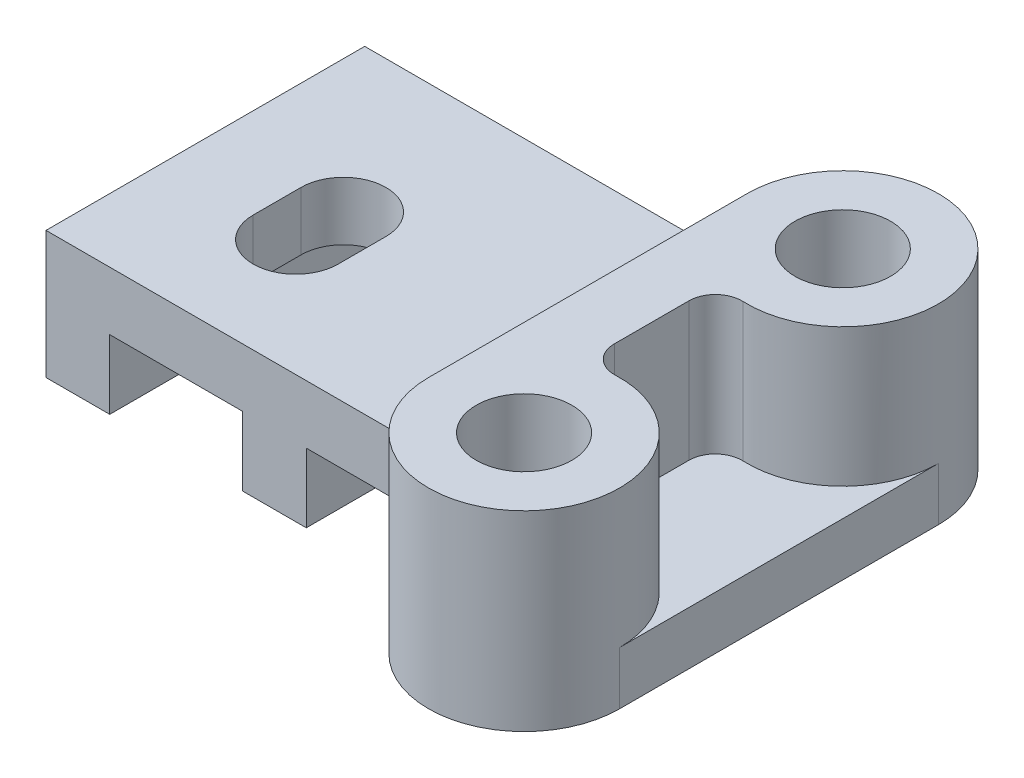
ISO-10303-21;
HEADER;
FILE_DESCRIPTION(('STEP AP214'),'2;1');
FILE_NAME('part.step','',(''),(''),'','','');
FILE_SCHEMA(('AUTOMOTIVE_DESIGN { 1 0 10303 214 1 1 1 1 }'));
ENDSEC;
DATA;
#1=APPLICATION_CONTEXT('core data for automotive mechanical design processes');
#2=APPLICATION_PROTOCOL_DEFINITION('international standard','automotive_design',2000,#1);
#3=PRODUCT_CONTEXT('',#1,'mechanical');
#4=PRODUCT('Part','Part','',(#3));
#5=PRODUCT_RELATED_PRODUCT_CATEGORY('part','',(#4));
#6=PRODUCT_DEFINITION_FORMATION('','',#4);
#7=PRODUCT_DEFINITION_CONTEXT('part definition',#1,'design');
#8=PRODUCT_DEFINITION('design','',#6,#7);
#9=PRODUCT_DEFINITION_SHAPE('','',#8);
#10=(LENGTH_UNIT() NAMED_UNIT(*) SI_UNIT(.MILLI.,.METRE.));
#11=(NAMED_UNIT(*) PLANE_ANGLE_UNIT() SI_UNIT($,.RADIAN.));
#12=(NAMED_UNIT(*) SI_UNIT($,.STERADIAN.) SOLID_ANGLE_UNIT());
#13=UNCERTAINTY_MEASURE_WITH_UNIT(LENGTH_MEASURE(1.E-05),#10,'distance_accuracy_value','');
#14=(GEOMETRIC_REPRESENTATION_CONTEXT(3) GLOBAL_UNCERTAINTY_ASSIGNED_CONTEXT((#13)) GLOBAL_UNIT_ASSIGNED_CONTEXT((#10,
#11,#12)) REPRESENTATION_CONTEXT('',''));
#15=CARTESIAN_POINT('',(0.,0.,0.));
#16=DIRECTION('',(0.,0.,1.));
#17=DIRECTION('',(1.,0.,0.));
#18=AXIS2_PLACEMENT_3D('',#15,#16,#17);
#19=CARTESIAN_POINT('',(90.,0.,0.));
#20=DIRECTION('',(0.,1.,0.));
#21=DIRECTION('',(0.,0.,1.));
#22=AXIS2_PLACEMENT_3D('',#19,#20,#21);
#23=CYLINDRICAL_SURFACE('',#22,18.);
#24=CARTESIAN_POINT('',(90.,10.,0.));
#25=DIRECTION('',(0.,1.,0.));
#26=DIRECTION('',(0.,0.,1.));
#27=AXIS2_PLACEMENT_3D('',#24,#25,#26);
#28=CIRCLE('',#27,18.);
#29=CARTESIAN_POINT('',(89.2173913043478,10.,17.9829787195973));
#30=VERTEX_POINT('',#29);
#31=CARTESIAN_POINT('',(108.,10.,0.));
#32=VERTEX_POINT('',#31);
#33=EDGE_CURVE('E236',#30,#32,#28,.T.);
#34=ORIENTED_EDGE('',*,*,#33,.T.);
#35=DIRECTION('',(0.,-1.,0.));
#36=VECTOR('',#35,1.);
#37=CARTESIAN_POINT('',(108.,10.,0.));
#38=LINE('',#37,#36);
#39=CARTESIAN_POINT('',(108.,0.,0.));
#40=VERTEX_POINT('',#39);
#41=EDGE_CURVE('E244',#32,#40,#38,.T.);
#42=ORIENTED_EDGE('',*,*,#41,.T.);
#43=CARTESIAN_POINT('',(90.,0.,0.));
#44=DIRECTION('',(0.,1.,0.));
#45=DIRECTION('',(0.,0.,1.));
#46=AXIS2_PLACEMENT_3D('',#43,#44,#45);
#47=CIRCLE('',#46,18.);
#48=CARTESIAN_POINT('',(72.,0.,0.));
#49=VERTEX_POINT('',#48);
#50=EDGE_CURVE('E264',#40,#49,#47,.T.);
#51=ORIENTED_EDGE('',*,*,#50,.T.);
#52=DIRECTION('',(0.,1.,0.));
#53=VECTOR('',#52,1.);
#54=CARTESIAN_POINT('',(72.,0.,0.));
#55=LINE('',#54,#53);
#56=CARTESIAN_POINT('',(72.,13.,0.));
#57=VERTEX_POINT('',#56);
#58=EDGE_CURVE('E303',#49,#57,#55,.T.);
#59=ORIENTED_EDGE('',*,*,#58,.T.);
#60=DIRECTION('',(0.,1.,0.));
#61=VECTOR('',#60,1.);
#62=CARTESIAN_POINT('',(72.,13.,0.));
#63=LINE('',#62,#61);
#64=CARTESIAN_POINT('',(72.,24.,0.));
#65=VERTEX_POINT('',#64);
#66=EDGE_CURVE('E344',#57,#65,#63,.T.);
#67=ORIENTED_EDGE('',*,*,#66,.T.);
#68=CARTESIAN_POINT('',(72.,36.,0.));
#69=VERTEX_POINT('',#68);
#70=EDGE_CURVE('E272',#65,#69,#55,.T.);
#71=ORIENTED_EDGE('',*,*,#70,.T.);
#72=CARTESIAN_POINT('',(90.,36.,0.));
#73=DIRECTION('',(0.,1.,0.));
#74=DIRECTION('',(0.,0.,1.));
#75=AXIS2_PLACEMENT_3D('',#72,#73,#74);
#76=CIRCLE('',#75,18.);
#77=CARTESIAN_POINT('',(89.2173913043478,36.,17.9829787195973));
#78=VERTEX_POINT('',#77);
#79=EDGE_CURVE('E265',#78,#69,#76,.T.);
#80=ORIENTED_EDGE('',*,*,#79,.F.);
#81=DIRECTION('',(0.,1.,0.));
#82=VECTOR('',#81,1.);
#83=CARTESIAN_POINT('',(89.2173913043478,0.,17.9829787195973));
#84=LINE('',#83,#82);
#85=EDGE_CURVE('E289',#30,#78,#84,.T.);
#86=ORIENTED_EDGE('',*,*,#85,.F.);
#87=EDGE_LOOP('',(#34,#42,#51,#59,#67,#71,#80,#86));
#88=FACE_BOUND('',#87,.T.);
#89=ADVANCED_FACE('F43',(#88),#23,.T.);
#90=CARTESIAN_POINT('',(0.,24.,60.));
#91=DIRECTION('',(1.,0.,0.));
#92=DIRECTION('',(0.,1.,0.));
#93=AXIS2_PLACEMENT_3D('',#90,#91,#92);
#94=PLANE('',#93);
#95=DIRECTION('',(0.,-1.,0.));
#96=VECTOR('',#95,1.);
#97=CARTESIAN_POINT('',(0.,24.,0.));
#98=LINE('',#97,#96);
#99=CARTESIAN_POINT('',(0.,24.,0.));
#100=VERTEX_POINT('',#99);
#101=CARTESIAN_POINT('',(0.,0.,0.));
#102=VERTEX_POINT('',#101);
#103=EDGE_CURVE('E295',#100,#102,#98,.T.);
#104=ORIENTED_EDGE('',*,*,#103,.T.);
#105=DIRECTION('',(0.,0.,-1.));
#106=VECTOR('',#105,1.);
#107=CARTESIAN_POINT('',(0.,0.,60.));
#108=LINE('',#107,#106);
#109=CARTESIAN_POINT('',(0.,0.,60.));
#110=VERTEX_POINT('',#109);
#111=EDGE_CURVE('E11',#110,#102,#108,.T.);
#112=ORIENTED_EDGE('',*,*,#111,.F.);
#113=DIRECTION('',(0.,-1.,0.));
#114=VECTOR('',#113,1.);
#115=CARTESIAN_POINT('',(0.,24.,60.));
#116=LINE('',#115,#114);
#117=CARTESIAN_POINT('',(0.,24.,60.));
#118=VERTEX_POINT('',#117);
#119=EDGE_CURVE('E308',#118,#110,#116,.T.);
#120=ORIENTED_EDGE('',*,*,#119,.F.);
#121=DIRECTION('',(0.,0.,-1.));
#122=VECTOR('',#121,1.);
#123=CARTESIAN_POINT('',(0.,24.,60.));
#124=LINE('',#123,#122);
#125=EDGE_CURVE('E327',#118,#100,#124,.T.);
#126=ORIENTED_EDGE('',*,*,#125,.T.);
#127=EDGE_LOOP('',(#104,#112,#120,#126));
#128=FACE_BOUND('',#127,.T.);
#129=ADVANCED_FACE('F44',(#128),#94,.F.);
#130=CARTESIAN_POINT('',(0.,0.,60.));
#131=DIRECTION('',(0.,1.,0.));
#132=DIRECTION('',(0.,0.,1.));
#133=AXIS2_PLACEMENT_3D('',#130,#131,#132);
#134=PLANE('',#133);
#135=DIRECTION('',(1.,0.,0.));
#136=VECTOR('',#135,1.);
#137=CARTESIAN_POINT('',(0.,0.,0.));
#138=LINE('',#137,#136);
#139=CARTESIAN_POINT('',(12.,0.,0.));
#140=VERTEX_POINT('',#139);
#141=EDGE_CURVE('E332',#102,#140,#138,.T.);
#142=ORIENTED_EDGE('',*,*,#141,.T.);
#143=DIRECTION('',(0.,0.,-1.));
#144=VECTOR('',#143,1.);
#145=CARTESIAN_POINT('',(12.,0.,60.));
#146=LINE('',#145,#144);
#147=CARTESIAN_POINT('',(12.,0.,60.));
#148=VERTEX_POINT('',#147);
#149=EDGE_CURVE('E51',#148,#140,#146,.T.);
#150=ORIENTED_EDGE('',*,*,#149,.F.);
#151=DIRECTION('',(1.,0.,0.));
#152=VECTOR('',#151,1.);
#153=CARTESIAN_POINT('',(0.,0.,60.));
#154=LINE('',#153,#152);
#155=EDGE_CURVE('E310',#110,#148,#154,.T.);
#156=ORIENTED_EDGE('',*,*,#155,.F.);
#157=ORIENTED_EDGE('',*,*,#111,.T.);
#158=EDGE_LOOP('',(#142,#150,#156,#157));
#159=FACE_BOUND('',#158,.T.);
#160=ADVANCED_FACE('F397',(#159),#134,.F.);
#161=CARTESIAN_POINT('',(12.,0.,60.));
#162=DIRECTION('',(-1.,0.,0.));
#163=DIRECTION('',(0.,0.,1.));
#164=AXIS2_PLACEMENT_3D('',#161,#162,#163);
#165=PLANE('',#164);
#166=DIRECTION('',(0.,1.,0.));
#167=VECTOR('',#166,1.);
#168=CARTESIAN_POINT('',(12.,0.,0.));
#169=LINE('',#168,#167);
#170=CARTESIAN_POINT('',(12.,13.,0.));
#171=VERTEX_POINT('',#170);
#172=EDGE_CURVE('E334',#140,#171,#169,.T.);
#173=ORIENTED_EDGE('',*,*,#172,.T.);
#174=DIRECTION('',(0.,0.,-1.));
#175=VECTOR('',#174,1.);
#176=CARTESIAN_POINT('',(12.,13.,60.));
#177=LINE('',#176,#175);
#178=CARTESIAN_POINT('',(12.,13.,60.));
#179=VERTEX_POINT('',#178);
#180=EDGE_CURVE('E369',#179,#171,#177,.T.);
#181=ORIENTED_EDGE('',*,*,#180,.F.);
#182=DIRECTION('',(0.,1.,0.));
#183=VECTOR('',#182,1.);
#184=CARTESIAN_POINT('',(12.,0.,60.));
#185=LINE('',#184,#183);
#186=EDGE_CURVE('E315',#148,#179,#185,.T.);
#187=ORIENTED_EDGE('',*,*,#186,.F.);
#188=ORIENTED_EDGE('',*,*,#149,.T.);
#189=EDGE_LOOP('',(#173,#181,#187,#188));
#190=FACE_BOUND('',#189,.T.);
#191=ADVANCED_FACE('F376',(#190),#165,.F.);
#192=CARTESIAN_POINT('',(12.,13.,60.));
#193=DIRECTION('',(0.,1.,0.));
#194=DIRECTION('',(0.,0.,1.));
#195=AXIS2_PLACEMENT_3D('',#192,#193,#194);
#196=PLANE('',#195);
#197=DIRECTION('',(0.,0.,-1.));
#198=VECTOR('',#197,1.);
#199=CARTESIAN_POINT('',(33.,13.,60.));
#200=LINE('',#199,#198);
#201=CARTESIAN_POINT('',(33.,13.,38.));
#202=VERTEX_POINT('',#201);
#203=CARTESIAN_POINT('',(33.,13.,29.));
#204=VERTEX_POINT('',#203);
#205=EDGE_CURVE('E224',#202,#204,#200,.T.);
#206=ORIENTED_EDGE('',*,*,#205,.T.);
#207=CARTESIAN_POINT('',(25.,13.,29.));
#208=DIRECTION('',(0.,1.,0.));
#209=DIRECTION('',(0.,0.,1.));
#210=AXIS2_PLACEMENT_3D('',#207,#208,#209);
#211=CIRCLE('',#210,8.00000000000001);
#212=CARTESIAN_POINT('',(17.,13.,29.));
#213=VERTEX_POINT('',#212);
#214=EDGE_CURVE('E228',#204,#213,#211,.T.);
#215=ORIENTED_EDGE('',*,*,#214,.T.);
#216=DIRECTION('',(0.,0.,1.));
#217=VECTOR('',#216,1.);
#218=CARTESIAN_POINT('',(17.,13.,60.));
#219=LINE('',#218,#217);
#220=CARTESIAN_POINT('',(17.,13.,38.));
#221=VERTEX_POINT('',#220);
#222=EDGE_CURVE('E217',#213,#221,#219,.T.);
#223=ORIENTED_EDGE('',*,*,#222,.T.);
#224=CARTESIAN_POINT('',(25.,13.,38.));
#225=DIRECTION('',(0.,1.,0.));
#226=DIRECTION('',(0.,0.,1.));
#227=AXIS2_PLACEMENT_3D('',#224,#225,#226);
#228=CIRCLE('',#227,8.);
#229=EDGE_CURVE('E196',#221,#202,#228,.T.);
#230=ORIENTED_EDGE('',*,*,#229,.T.);
#231=EDGE_LOOP('',(#206,#215,#223,#230));
#232=FACE_BOUND('',#231,.T.);
#233=DIRECTION('',(1.,0.,0.));
#234=VECTOR('',#233,1.);
#235=CARTESIAN_POINT('',(12.,13.,0.));
#236=LINE('',#235,#234);
#237=CARTESIAN_POINT('',(37.,13.,0.));
#238=VERTEX_POINT('',#237);
#239=EDGE_CURVE('E333',#171,#238,#236,.T.);
#240=ORIENTED_EDGE('',*,*,#239,.T.);
#241=DIRECTION('',(0.,0.,-1.));
#242=VECTOR('',#241,1.);
#243=CARTESIAN_POINT('',(37.,13.,60.));
#244=LINE('',#243,#242);
#245=CARTESIAN_POINT('',(37.,13.,60.));
#246=VERTEX_POINT('',#245);
#247=EDGE_CURVE('E368',#246,#238,#244,.T.);
#248=ORIENTED_EDGE('',*,*,#247,.F.);
#249=DIRECTION('',(1.,0.,0.));
#250=VECTOR('',#249,1.);
#251=CARTESIAN_POINT('',(12.,13.,60.));
#252=LINE('',#251,#250);
#253=EDGE_CURVE('E314',#179,#246,#252,.T.);
#254=ORIENTED_EDGE('',*,*,#253,.F.);
#255=ORIENTED_EDGE('',*,*,#180,.T.);
#256=EDGE_LOOP('',(#240,#248,#254,#255));
#257=FACE_BOUND('',#256,.T.);
#258=ADVANCED_FACE('F390',(#232,#257),#196,.F.);
#259=CARTESIAN_POINT('',(37.,13.,60.));
#260=DIRECTION('',(1.,0.,0.));
#261=DIRECTION('',(0.,0.,-1.));
#262=AXIS2_PLACEMENT_3D('',#259,#260,#261);
#263=PLANE('',#262);
#264=DIRECTION('',(0.,-1.,0.));
#265=VECTOR('',#264,1.);
#266=CARTESIAN_POINT('',(37.,13.,0.));
#267=LINE('',#266,#265);
#268=CARTESIAN_POINT('',(37.,0.,0.));
#269=VERTEX_POINT('',#268);
#270=EDGE_CURVE('E339',#238,#269,#267,.T.);
#271=ORIENTED_EDGE('',*,*,#270,.T.);
#272=DIRECTION('',(0.,0.,-1.));
#273=VECTOR('',#272,1.);
#274=CARTESIAN_POINT('',(37.,0.,60.));
#275=LINE('',#274,#273);
#276=CARTESIAN_POINT('',(37.,0.,60.));
#277=VERTEX_POINT('',#276);
#278=EDGE_CURVE('E361',#277,#269,#275,.T.);
#279=ORIENTED_EDGE('',*,*,#278,.F.);
#280=DIRECTION('',(0.,-1.,0.));
#281=VECTOR('',#280,1.);
#282=CARTESIAN_POINT('',(37.,13.,60.));
#283=LINE('',#282,#281);
#284=EDGE_CURVE('E316',#246,#277,#283,.T.);
#285=ORIENTED_EDGE('',*,*,#284,.F.);
#286=ORIENTED_EDGE('',*,*,#247,.T.);
#287=EDGE_LOOP('',(#271,#279,#285,#286));
#288=FACE_BOUND('',#287,.T.);
#289=ADVANCED_FACE('F393',(#288),#263,.F.);
#290=CARTESIAN_POINT('',(37.,0.,60.));
#291=DIRECTION('',(0.,1.,0.));
#292=DIRECTION('',(0.,0.,1.));
#293=AXIS2_PLACEMENT_3D('',#290,#291,#292);
#294=PLANE('',#293);
#295=DIRECTION('',(1.,0.,0.));
#296=VECTOR('',#295,1.);
#297=CARTESIAN_POINT('',(37.,0.,0.));
#298=LINE('',#297,#296);
#299=CARTESIAN_POINT('',(49.,0.,0.));
#300=VERTEX_POINT('',#299);
#301=EDGE_CURVE('E340',#269,#300,#298,.T.);
#302=ORIENTED_EDGE('',*,*,#301,.T.);
#303=DIRECTION('',(0.,0.,-1.));
#304=VECTOR('',#303,1.);
#305=CARTESIAN_POINT('',(49.,0.,60.));
#306=LINE('',#305,#304);
#307=CARTESIAN_POINT('',(49.,0.,60.));
#308=VERTEX_POINT('',#307);
#309=EDGE_CURVE('E359',#308,#300,#306,.T.);
#310=ORIENTED_EDGE('',*,*,#309,.F.);
#311=DIRECTION('',(1.,0.,0.));
#312=VECTOR('',#311,1.);
#313=CARTESIAN_POINT('',(37.,0.,60.));
#314=LINE('',#313,#312);
#315=EDGE_CURVE('E318',#277,#308,#314,.T.);
#316=ORIENTED_EDGE('',*,*,#315,.F.);
#317=ORIENTED_EDGE('',*,*,#278,.T.);
#318=EDGE_LOOP('',(#302,#310,#316,#317));
#319=FACE_BOUND('',#318,.T.);
#320=ADVANCED_FACE('F452',(#319),#294,.F.);
#321=CARTESIAN_POINT('',(49.,0.,60.));
#322=DIRECTION('',(-1.,0.,0.));
#323=DIRECTION('',(0.,0.,1.));
#324=AXIS2_PLACEMENT_3D('',#321,#322,#323);
#325=PLANE('',#324);
#326=DIRECTION('',(0.,1.,0.));
#327=VECTOR('',#326,1.);
#328=CARTESIAN_POINT('',(49.,0.,0.));
#329=LINE('',#328,#327);
#330=CARTESIAN_POINT('',(49.,13.,0.));
#331=VERTEX_POINT('',#330);
#332=EDGE_CURVE('E341',#300,#331,#329,.T.);
#333=ORIENTED_EDGE('',*,*,#332,.T.);
#334=DIRECTION('',(0.,0.,-1.));
#335=VECTOR('',#334,1.);
#336=CARTESIAN_POINT('',(49.,13.,60.));
#337=LINE('',#336,#335);
#338=CARTESIAN_POINT('',(49.,13.,60.));
#339=VERTEX_POINT('',#338);
#340=EDGE_CURVE('E360',#339,#331,#337,.T.);
#341=ORIENTED_EDGE('',*,*,#340,.F.);
#342=DIRECTION('',(0.,1.,0.));
#343=VECTOR('',#342,1.);
#344=CARTESIAN_POINT('',(49.,0.,60.));
#345=LINE('',#344,#343);
#346=EDGE_CURVE('E319',#308,#339,#345,.T.);
#347=ORIENTED_EDGE('',*,*,#346,.F.);
#348=ORIENTED_EDGE('',*,*,#309,.T.);
#349=EDGE_LOOP('',(#333,#341,#347,#348));
#350=FACE_BOUND('',#349,.T.);
#351=ADVANCED_FACE('F455',(#350),#325,.F.);
#352=CARTESIAN_POINT('',(49.,13.,60.));
#353=DIRECTION('',(0.,1.,0.));
#354=DIRECTION('',(0.,0.,1.));
#355=AXIS2_PLACEMENT_3D('',#352,#353,#354);
#356=PLANE('',#355);
#357=DIRECTION('',(1.,0.,0.));
#358=VECTOR('',#357,1.);
#359=CARTESIAN_POINT('',(49.,13.,0.));
#360=LINE('',#359,#358);
#361=EDGE_CURVE('E343',#331,#57,#360,.T.);
#362=ORIENTED_EDGE('',*,*,#361,.T.);
#363=DIRECTION('',(0.,0.,-1.));
#364=VECTOR('',#363,1.);
#365=CARTESIAN_POINT('',(72.,13.,60.));
#366=LINE('',#365,#364);
#367=CARTESIAN_POINT('',(72.,13.,60.));
#368=VERTEX_POINT('',#367);
#369=EDGE_CURVE('E355',#368,#57,#366,.T.);
#370=ORIENTED_EDGE('',*,*,#369,.F.);
#371=DIRECTION('',(1.,0.,0.));
#372=VECTOR('',#371,1.);
#373=CARTESIAN_POINT('',(49.,13.,60.));
#374=LINE('',#373,#372);
#375=EDGE_CURVE('E325',#339,#368,#374,.T.);
#376=ORIENTED_EDGE('',*,*,#375,.F.);
#377=ORIENTED_EDGE('',*,*,#340,.T.);
#378=EDGE_LOOP('',(#362,#370,#376,#377));
#379=FACE_BOUND('',#378,.T.);
#380=ADVANCED_FACE('F450',(#379),#356,.F.);
#381=CARTESIAN_POINT('',(72.,24.,60.));
#382=DIRECTION('',(0.,-1.,0.));
#383=DIRECTION('',(1.,0.,0.));
#384=AXIS2_PLACEMENT_3D('',#381,#382,#383);
#385=PLANE('',#384);
#386=DIRECTION('',(0.,0.,1.));
#387=VECTOR('',#386,1.);
#388=CARTESIAN_POINT('',(17.,24.,29.));
#389=LINE('',#388,#387);
#390=CARTESIAN_POINT('',(17.,24.,29.));
#391=VERTEX_POINT('',#390);
#392=CARTESIAN_POINT('',(17.,24.,38.));
#393=VERTEX_POINT('',#392);
#394=EDGE_CURVE('E204',#391,#393,#389,.T.);
#395=ORIENTED_EDGE('',*,*,#394,.F.);
#396=CARTESIAN_POINT('',(25.,24.,29.));
#397=DIRECTION('',(0.,1.,0.));
#398=DIRECTION('',(-1.,0.,0.));
#399=AXIS2_PLACEMENT_3D('',#396,#397,#398);
#400=CIRCLE('',#399,8.00000000000001);
#401=CARTESIAN_POINT('',(33.,24.,29.));
#402=VERTEX_POINT('',#401);
#403=EDGE_CURVE('E66',#402,#391,#400,.T.);
#404=ORIENTED_EDGE('',*,*,#403,.F.);
#405=DIRECTION('',(0.,0.,-1.));
#406=VECTOR('',#405,1.);
#407=CARTESIAN_POINT('',(33.,24.,29.));
#408=LINE('',#407,#406);
#409=CARTESIAN_POINT('',(33.,24.,38.));
#410=VERTEX_POINT('',#409);
#411=EDGE_CURVE('E211',#410,#402,#408,.T.);
#412=ORIENTED_EDGE('',*,*,#411,.F.);
#413=CARTESIAN_POINT('',(25.,24.,38.));
#414=DIRECTION('',(0.,1.,0.));
#415=DIRECTION('',(-1.,0.,0.));
#416=AXIS2_PLACEMENT_3D('',#413,#414,#415);
#417=CIRCLE('',#416,8.);
#418=EDGE_CURVE('E194',#393,#410,#417,.T.);
#419=ORIENTED_EDGE('',*,*,#418,.F.);
#420=EDGE_LOOP('',(#395,#404,#412,#419));
#421=FACE_BOUND('',#420,.T.);
#422=DIRECTION('',(-1.,0.,0.));
#423=VECTOR('',#422,1.);
#424=CARTESIAN_POINT('',(72.,24.,0.));
#425=LINE('',#424,#423);
#426=EDGE_CURVE('E309',#65,#100,#425,.T.);
#427=ORIENTED_EDGE('',*,*,#426,.T.);
#428=ORIENTED_EDGE('',*,*,#125,.F.);
#429=DIRECTION('',(-1.,0.,0.));
#430=VECTOR('',#429,1.);
#431=CARTESIAN_POINT('',(72.,24.,60.));
#432=LINE('',#431,#430);
#433=CARTESIAN_POINT('',(72.,24.,60.));
#434=VERTEX_POINT('',#433);
#435=EDGE_CURVE('E326',#434,#118,#432,.T.);
#436=ORIENTED_EDGE('',*,*,#435,.F.);
#437=DIRECTION('',(0.,0.,-1.));
#438=VECTOR('',#437,1.);
#439=CARTESIAN_POINT('',(72.,24.,60.));
#440=LINE('',#439,#438);
#441=EDGE_CURVE('E353',#434,#65,#440,.T.);
#442=ORIENTED_EDGE('',*,*,#441,.T.);
#443=EDGE_LOOP('',(#427,#428,#436,#442));
#444=FACE_BOUND('',#443,.T.);
#445=ADVANCED_FACE('F208',(#421,#444),#385,.F.);
#446=CARTESIAN_POINT('',(0.,0.,60.));
#447=DIRECTION('',(0.,0.,1.));
#448=DIRECTION('',(1.,0.,0.));
#449=AXIS2_PLACEMENT_3D('',#446,#447,#448);
#450=PLANE('',#449);
#451=ORIENTED_EDGE('',*,*,#119,.T.);
#452=ORIENTED_EDGE('',*,*,#155,.T.);
#453=ORIENTED_EDGE('',*,*,#186,.T.);
#454=ORIENTED_EDGE('',*,*,#253,.T.);
#455=ORIENTED_EDGE('',*,*,#284,.T.);
#456=ORIENTED_EDGE('',*,*,#315,.T.);
#457=ORIENTED_EDGE('',*,*,#346,.T.);
#458=ORIENTED_EDGE('',*,*,#375,.T.);
#459=DIRECTION('',(0.,1.,0.));
#460=VECTOR('',#459,1.);
#461=CARTESIAN_POINT('',(72.,13.,60.));
#462=LINE('',#461,#460);
#463=EDGE_CURVE('E322',#368,#434,#462,.T.);
#464=ORIENTED_EDGE('',*,*,#463,.T.);
#465=ORIENTED_EDGE('',*,*,#435,.T.);
#466=EDGE_LOOP('',(#451,#452,#453,#454,#455,#456,#457,#458,#464,#465));
#467=FACE_BOUND('',#466,.T.);
#468=ADVANCED_FACE('F391',(#467),#450,.T.);
#469=CARTESIAN_POINT('',(0.,0.,0.));
#470=DIRECTION('',(0.,0.,1.));
#471=DIRECTION('',(1.,0.,0.));
#472=AXIS2_PLACEMENT_3D('',#469,#470,#471);
#473=PLANE('',#472);
#474=ORIENTED_EDGE('',*,*,#103,.F.);
#475=ORIENTED_EDGE('',*,*,#426,.F.);
#476=ORIENTED_EDGE('',*,*,#66,.F.);
#477=ORIENTED_EDGE('',*,*,#361,.F.);
#478=ORIENTED_EDGE('',*,*,#332,.F.);
#479=ORIENTED_EDGE('',*,*,#301,.F.);
#480=ORIENTED_EDGE('',*,*,#270,.F.);
#481=ORIENTED_EDGE('',*,*,#239,.F.);
#482=ORIENTED_EDGE('',*,*,#172,.F.);
#483=ORIENTED_EDGE('',*,*,#141,.F.);
#484=EDGE_LOOP('',(#474,#475,#476,#477,#478,#479,#480,#481,#482,#483));
#485=FACE_BOUND('',#484,.T.);
#486=ADVANCED_FACE('F385',(#485),#473,.F.);
#487=CARTESIAN_POINT('',(72.,0.,0.));
#488=DIRECTION('',(-1.,0.,0.));
#489=DIRECTION('',(0.,0.,1.));
#490=AXIS2_PLACEMENT_3D('',#487,#488,#489);
#491=PLANE('',#490);
#492=ORIENTED_EDGE('',*,*,#369,.T.);
#493=ORIENTED_EDGE('',*,*,#58,.F.);
#494=DIRECTION('',(0.,0.,1.));
#495=VECTOR('',#494,1.);
#496=CARTESIAN_POINT('',(72.,0.,0.));
#497=LINE('',#496,#495);
#498=CARTESIAN_POINT('',(72.,0.,60.));
#499=VERTEX_POINT('',#498);
#500=EDGE_CURVE('E270',#49,#499,#497,.T.);
#501=ORIENTED_EDGE('',*,*,#500,.T.);
#502=DIRECTION('',(0.,1.,0.));
#503=VECTOR('',#502,1.);
#504=CARTESIAN_POINT('',(72.,0.,60.));
#505=LINE('',#504,#503);
#506=EDGE_CURVE('E300',#499,#368,#505,.T.);
#507=ORIENTED_EDGE('',*,*,#506,.T.);
#508=EDGE_LOOP('',(#492,#493,#501,#507));
#509=FACE_BOUND('',#508,.T.);
#510=ADVANCED_FACE('F417',(#509),#491,.T.);
#511=ORIENTED_EDGE('',*,*,#441,.F.);
#512=CARTESIAN_POINT('',(72.,36.,60.));
#513=VERTEX_POINT('',#512);
#514=EDGE_CURVE('E305',#434,#513,#505,.T.);
#515=ORIENTED_EDGE('',*,*,#514,.T.);
#516=DIRECTION('',(0.,0.,1.));
#517=VECTOR('',#516,1.);
#518=CARTESIAN_POINT('',(72.,36.,0.));
#519=LINE('',#518,#517);
#520=EDGE_CURVE('E277',#69,#513,#519,.T.);
#521=ORIENTED_EDGE('',*,*,#520,.F.);
#522=ORIENTED_EDGE('',*,*,#70,.F.);
#523=EDGE_LOOP('',(#511,#515,#521,#522));
#524=FACE_BOUND('',#523,.T.);
#525=ADVANCED_FACE('F406',(#524),#491,.T.);
#526=CARTESIAN_POINT('',(89.,0.,22.9782505861521));
#527=DIRECTION('',(0.,1.,0.));
#528=DIRECTION('',(0.,0.,1.));
#529=AXIS2_PLACEMENT_3D('',#526,#527,#528);
#530=CYLINDRICAL_SURFACE('',#529,5.);
#531=CARTESIAN_POINT('',(89.,10.,22.9782505861521));
#532=DIRECTION('',(0.,1.,0.));
#533=DIRECTION('',(0.,0.,1.));
#534=AXIS2_PLACEMENT_3D('',#531,#532,#533);
#535=CIRCLE('',#534,5.00000000000001);
#536=CARTESIAN_POINT('',(84.,10.,22.9782505861521));
#537=VERTEX_POINT('',#536);
#538=EDGE_CURVE('E238',#537,#30,#535,.F.);
#539=ORIENTED_EDGE('',*,*,#538,.T.);
#540=ORIENTED_EDGE('',*,*,#85,.T.);
#541=CARTESIAN_POINT('',(89.,36.,22.9782505861521));
#542=DIRECTION('',(0.,-1.,0.));
#543=DIRECTION('',(0.,0.,1.));
#544=AXIS2_PLACEMENT_3D('',#541,#542,#543);
#545=CIRCLE('',#544,5.);
#546=CARTESIAN_POINT('',(84.,36.,22.9782505861521));
#547=VERTEX_POINT('',#546);
#548=EDGE_CURVE('E268',#547,#78,#545,.T.);
#549=ORIENTED_EDGE('',*,*,#548,.F.);
#550=DIRECTION('',(0.,1.,0.));
#551=VECTOR('',#550,1.);
#552=CARTESIAN_POINT('',(84.,0.,22.9782505861521));
#553=LINE('',#552,#551);
#554=EDGE_CURVE('E291',#537,#547,#553,.T.);
#555=ORIENTED_EDGE('',*,*,#554,.F.);
#556=EDGE_LOOP('',(#539,#540,#549,#555));
#557=FACE_BOUND('',#556,.T.);
#558=ADVANCED_FACE('F508',(#557),#530,.F.);
#559=CARTESIAN_POINT('',(84.,0.,22.9782505861521));
#560=DIRECTION('',(1.,0.,0.));
#561=DIRECTION('',(0.,0.,-1.));
#562=AXIS2_PLACEMENT_3D('',#559,#560,#561);
#563=PLANE('',#562);
#564=DIRECTION('',(0.,0.,1.));
#565=VECTOR('',#564,1.);
#566=CARTESIAN_POINT('',(84.,10.,0.));
#567=LINE('',#566,#565);
#568=CARTESIAN_POINT('',(84.,10.,37.0217494138479));
#569=VERTEX_POINT('',#568);
#570=EDGE_CURVE('E226',#537,#569,#567,.T.);
#571=ORIENTED_EDGE('',*,*,#570,.F.);
#572=ORIENTED_EDGE('',*,*,#554,.T.);
#573=DIRECTION('',(0.,0.,-1.));
#574=VECTOR('',#573,1.);
#575=CARTESIAN_POINT('',(84.,36.,22.9782505861521));
#576=LINE('',#575,#574);
#577=CARTESIAN_POINT('',(84.,36.,37.0217494138479));
#578=VERTEX_POINT('',#577);
#579=EDGE_CURVE('E281',#578,#547,#576,.T.);
#580=ORIENTED_EDGE('',*,*,#579,.F.);
#581=DIRECTION('',(0.,1.,0.));
#582=VECTOR('',#581,1.);
#583=CARTESIAN_POINT('',(84.,0.,37.0217494138479));
#584=LINE('',#583,#582);
#585=EDGE_CURVE('E293',#569,#578,#584,.T.);
#586=ORIENTED_EDGE('',*,*,#585,.F.);
#587=EDGE_LOOP('',(#571,#572,#580,#586));
#588=FACE_BOUND('',#587,.T.);
#589=ADVANCED_FACE('F609',(#588),#563,.T.);
#590=CARTESIAN_POINT('',(89.,0.,37.0217494138479));
#591=DIRECTION('',(0.,1.,0.));
#592=DIRECTION('',(0.,0.,1.));
#593=AXIS2_PLACEMENT_3D('',#590,#591,#592);
#594=CYLINDRICAL_SURFACE('',#593,5.00000000000001);
#595=CARTESIAN_POINT('',(89.,10.,37.0217494138479));
#596=DIRECTION('',(0.,1.,0.));
#597=DIRECTION('',(0.,0.,1.));
#598=AXIS2_PLACEMENT_3D('',#595,#596,#597);
#599=CIRCLE('',#598,5.00000000000001);
#600=CARTESIAN_POINT('',(89.2173913043479,10.,42.0170212804027));
#601=VERTEX_POINT('',#600);
#602=EDGE_CURVE('E247',#569,#601,#599,.T.);
#603=ORIENTED_EDGE('',*,*,#602,.F.);
#604=ORIENTED_EDGE('',*,*,#585,.T.);
#605=CARTESIAN_POINT('',(89.,36.,37.0217494138479));
#606=DIRECTION('',(0.,-1.,0.));
#607=DIRECTION('',(0.,0.,1.));
#608=AXIS2_PLACEMENT_3D('',#605,#606,#607);
#609=CIRCLE('',#608,5.00000000000001);
#610=CARTESIAN_POINT('',(89.2173913043479,36.,42.0170212804027));
#611=VERTEX_POINT('',#610);
#612=EDGE_CURVE('E284',#611,#578,#609,.T.);
#613=ORIENTED_EDGE('',*,*,#612,.F.);
#614=DIRECTION('',(0.,1.,0.));
#615=VECTOR('',#614,1.);
#616=CARTESIAN_POINT('',(89.2173913043479,0.,42.0170212804027));
#617=LINE('',#616,#615);
#618=EDGE_CURVE('E299',#601,#611,#617,.T.);
#619=ORIENTED_EDGE('',*,*,#618,.F.);
#620=EDGE_LOOP('',(#603,#604,#613,#619));
#621=FACE_BOUND('',#620,.T.);
#622=ADVANCED_FACE('F439',(#621),#594,.F.);
#623=CARTESIAN_POINT('',(90.,0.,60.));
#624=DIRECTION('',(0.,1.,0.));
#625=DIRECTION('',(0.,0.,1.));
#626=AXIS2_PLACEMENT_3D('',#623,#624,#625);
#627=CYLINDRICAL_SURFACE('',#626,18.);
#628=DIRECTION('',(0.,-1.,0.));
#629=VECTOR('',#628,1.);
#630=CARTESIAN_POINT('',(108.,10.,60.));
#631=LINE('',#630,#629);
#632=CARTESIAN_POINT('',(108.,10.,60.));
#633=VERTEX_POINT('',#632);
#634=CARTESIAN_POINT('',(108.,0.,60.));
#635=VERTEX_POINT('',#634);
#636=EDGE_CURVE('E246',#633,#635,#631,.T.);
#637=ORIENTED_EDGE('',*,*,#636,.F.);
#638=CARTESIAN_POINT('',(90.,10.,60.));
#639=DIRECTION('',(0.,1.,0.));
#640=DIRECTION('',(0.,0.,1.));
#641=AXIS2_PLACEMENT_3D('',#638,#639,#640);
#642=CIRCLE('',#641,18.);
#643=EDGE_CURVE('E233',#633,#601,#642,.T.);
#644=ORIENTED_EDGE('',*,*,#643,.T.);
#645=ORIENTED_EDGE('',*,*,#618,.T.);
#646=CARTESIAN_POINT('',(90.,36.,60.));
#647=DIRECTION('',(0.,1.,0.));
#648=DIRECTION('',(0.,0.,1.));
#649=AXIS2_PLACEMENT_3D('',#646,#647,#648);
#650=CIRCLE('',#649,18.);
#651=EDGE_CURVE('E276',#513,#611,#650,.T.);
#652=ORIENTED_EDGE('',*,*,#651,.F.);
#653=ORIENTED_EDGE('',*,*,#514,.F.);
#654=ORIENTED_EDGE('',*,*,#463,.F.);
#655=ORIENTED_EDGE('',*,*,#506,.F.);
#656=CARTESIAN_POINT('',(90.,0.,60.));
#657=DIRECTION('',(0.,1.,0.));
#658=DIRECTION('',(0.,0.,1.));
#659=AXIS2_PLACEMENT_3D('',#656,#657,#658);
#660=CIRCLE('',#659,18.);
#661=EDGE_CURVE('E271',#499,#635,#660,.T.);
#662=ORIENTED_EDGE('',*,*,#661,.T.);
#663=EDGE_LOOP('',(#637,#644,#645,#652,#653,#654,#655,#662));
#664=FACE_BOUND('',#663,.T.);
#665=ADVANCED_FACE('F422',(#664),#627,.T.);
#666=CARTESIAN_POINT('',(90.,0.,0.));
#667=DIRECTION('',(0.,1.,0.));
#668=DIRECTION('',(0.,0.,1.));
#669=AXIS2_PLACEMENT_3D('',#666,#667,#668);
#670=PLANE('',#669);
#671=ORIENTED_EDGE('',*,*,#50,.F.);
#672=DIRECTION('',(0.,0.,1.));
#673=VECTOR('',#672,1.);
#674=CARTESIAN_POINT('',(108.,0.,0.));
#675=LINE('',#674,#673);
#676=EDGE_CURVE('E230',#40,#635,#675,.T.);
#677=ORIENTED_EDGE('',*,*,#676,.T.);
#678=ORIENTED_EDGE('',*,*,#661,.F.);
#679=ORIENTED_EDGE('',*,*,#500,.F.);
#680=EDGE_LOOP('',(#671,#677,#678,#679));
#681=FACE_BOUND('',#680,.T.);
#682=CARTESIAN_POINT('',(90.,0.,60.));
#683=DIRECTION('',(0.,1.,0.));
#684=DIRECTION('',(0.,0.,1.));
#685=AXIS2_PLACEMENT_3D('',#682,#683,#684);
#686=CIRCLE('',#685,9.);
#687=CARTESIAN_POINT('',(90.,0.,69.));
#688=VERTEX_POINT('',#687);
#689=EDGE_CURVE('E259',#688,#688,#686,.T.);
#690=ORIENTED_EDGE('',*,*,#689,.T.);
#691=EDGE_LOOP('',(#690));
#692=FACE_BOUND('',#691,.T.);
#693=CARTESIAN_POINT('',(90.,0.,0.));
#694=DIRECTION('',(0.,1.,0.));
#695=DIRECTION('',(0.,0.,1.));
#696=AXIS2_PLACEMENT_3D('',#693,#694,#695);
#697=CIRCLE('',#696,9.);
#698=CARTESIAN_POINT('',(90.,0.,9.));
#699=VERTEX_POINT('',#698);
#700=EDGE_CURVE('E251',#699,#699,#697,.T.);
#701=ORIENTED_EDGE('',*,*,#700,.T.);
#702=EDGE_LOOP('',(#701));
#703=FACE_BOUND('',#702,.T.);
#704=ADVANCED_FACE('F423',(#681,#692,#703),#670,.F.);
#705=CARTESIAN_POINT('',(90.,36.,0.));
#706=DIRECTION('',(0.,1.,0.));
#707=DIRECTION('',(0.,0.,1.));
#708=AXIS2_PLACEMENT_3D('',#705,#706,#707);
#709=PLANE('',#708);
#710=CARTESIAN_POINT('',(90.,36.,0.));
#711=DIRECTION('',(0.,1.,0.));
#712=DIRECTION('',(0.,0.,1.));
#713=AXIS2_PLACEMENT_3D('',#710,#711,#712);
#714=CIRCLE('',#713,9.);
#715=CARTESIAN_POINT('',(90.,36.,9.));
#716=VERTEX_POINT('',#715);
#717=EDGE_CURVE('E252',#716,#716,#714,.T.);
#718=ORIENTED_EDGE('',*,*,#717,.F.);
#719=EDGE_LOOP('',(#718));
#720=FACE_BOUND('',#719,.T.);
#721=CARTESIAN_POINT('',(90.,36.,60.));
#722=DIRECTION('',(0.,1.,0.));
#723=DIRECTION('',(0.,0.,1.));
#724=AXIS2_PLACEMENT_3D('',#721,#722,#723);
#725=CIRCLE('',#724,9.);
#726=CARTESIAN_POINT('',(90.,36.,69.));
#727=VERTEX_POINT('',#726);
#728=EDGE_CURVE('E258',#727,#727,#725,.T.);
#729=ORIENTED_EDGE('',*,*,#728,.F.);
#730=EDGE_LOOP('',(#729));
#731=FACE_BOUND('',#730,.T.);
#732=ORIENTED_EDGE('',*,*,#79,.T.);
#733=ORIENTED_EDGE('',*,*,#520,.T.);
#734=ORIENTED_EDGE('',*,*,#651,.T.);
#735=ORIENTED_EDGE('',*,*,#612,.T.);
#736=ORIENTED_EDGE('',*,*,#579,.T.);
#737=ORIENTED_EDGE('',*,*,#548,.T.);
#738=EDGE_LOOP('',(#732,#733,#734,#735,#736,#737));
#739=FACE_BOUND('',#738,.T.);
#740=ADVANCED_FACE('F441',(#720,#731,#739),#709,.T.);
#741=CARTESIAN_POINT('',(90.,0.,60.));
#742=DIRECTION('',(0.,1.,0.));
#743=DIRECTION('',(0.,0.,1.));
#744=AXIS2_PLACEMENT_3D('',#741,#742,#743);
#745=CYLINDRICAL_SURFACE('',#744,9.);
#746=ORIENTED_EDGE('',*,*,#689,.F.);
#747=EDGE_LOOP('',(#746));
#748=FACE_BOUND('',#747,.T.);
#749=ORIENTED_EDGE('',*,*,#728,.T.);
#750=EDGE_LOOP('',(#749));
#751=FACE_BOUND('',#750,.T.);
#752=ADVANCED_FACE('F518',(#748,#751),#745,.F.);
#753=CARTESIAN_POINT('',(90.,0.,0.));
#754=DIRECTION('',(0.,1.,0.));
#755=DIRECTION('',(0.,0.,1.));
#756=AXIS2_PLACEMENT_3D('',#753,#754,#755);
#757=CYLINDRICAL_SURFACE('',#756,9.);
#758=ORIENTED_EDGE('',*,*,#700,.F.);
#759=EDGE_LOOP('',(#758));
#760=FACE_BOUND('',#759,.T.);
#761=ORIENTED_EDGE('',*,*,#717,.T.);
#762=EDGE_LOOP('',(#761));
#763=FACE_BOUND('',#762,.T.);
#764=ADVANCED_FACE('F524',(#760,#763),#757,.F.);
#765=CARTESIAN_POINT('',(108.,10.,0.));
#766=DIRECTION('',(1.,0.,0.));
#767=DIRECTION('',(0.,0.,-1.));
#768=AXIS2_PLACEMENT_3D('',#765,#766,#767);
#769=PLANE('',#768);
#770=ORIENTED_EDGE('',*,*,#676,.F.);
#771=ORIENTED_EDGE('',*,*,#41,.F.);
#772=DIRECTION('',(0.,0.,1.));
#773=VECTOR('',#772,1.);
#774=CARTESIAN_POINT('',(108.,10.,0.));
#775=LINE('',#774,#773);
#776=EDGE_CURVE('E234',#32,#633,#775,.T.);
#777=ORIENTED_EDGE('',*,*,#776,.T.);
#778=ORIENTED_EDGE('',*,*,#636,.T.);
#779=EDGE_LOOP('',(#770,#771,#777,#778));
#780=FACE_BOUND('',#779,.T.);
#781=ADVANCED_FACE('F427',(#780),#769,.T.);
#782=CARTESIAN_POINT('',(0.,10.,0.));
#783=DIRECTION('',(0.,1.,0.));
#784=DIRECTION('',(0.,0.,1.));
#785=AXIS2_PLACEMENT_3D('',#782,#783,#784);
#786=PLANE('',#785);
#787=ORIENTED_EDGE('',*,*,#570,.T.);
#788=ORIENTED_EDGE('',*,*,#602,.T.);
#789=ORIENTED_EDGE('',*,*,#643,.F.);
#790=ORIENTED_EDGE('',*,*,#776,.F.);
#791=ORIENTED_EDGE('',*,*,#33,.F.);
#792=ORIENTED_EDGE('',*,*,#538,.F.);
#793=EDGE_LOOP('',(#787,#788,#789,#790,#791,#792));
#794=FACE_BOUND('',#793,.T.);
#795=ADVANCED_FACE('F432',(#794),#786,.T.);
#796=CARTESIAN_POINT('',(25.,0.,29.));
#797=DIRECTION('',(0.,1.,0.));
#798=DIRECTION('',(-1.,0.,0.));
#799=AXIS2_PLACEMENT_3D('',#796,#797,#798);
#800=CYLINDRICAL_SURFACE('',#799,8.00000000000001);
#801=DIRECTION('',(0.,1.,0.));
#802=VECTOR('',#801,1.);
#803=CARTESIAN_POINT('',(33.,0.,29.));
#804=LINE('',#803,#802);
#805=EDGE_CURVE('E216',#204,#402,#804,.T.);
#806=ORIENTED_EDGE('',*,*,#805,.T.);
#807=ORIENTED_EDGE('',*,*,#403,.T.);
#808=DIRECTION('',(0.,1.,0.));
#809=VECTOR('',#808,1.);
#810=CARTESIAN_POINT('',(17.,0.,29.));
#811=LINE('',#810,#809);
#812=EDGE_CURVE('E203',#213,#391,#811,.T.);
#813=ORIENTED_EDGE('',*,*,#812,.F.);
#814=ORIENTED_EDGE('',*,*,#214,.F.);
#815=EDGE_LOOP('',(#806,#807,#813,#814));
#816=FACE_BOUND('',#815,.T.);
#817=ADVANCED_FACE('F566',(#816),#800,.F.);
#818=CARTESIAN_POINT('',(33.,0.,29.));
#819=DIRECTION('',(1.,0.,0.));
#820=DIRECTION('',(0.,0.,-1.));
#821=AXIS2_PLACEMENT_3D('',#818,#819,#820);
#822=PLANE('',#821);
#823=DIRECTION('',(0.,1.,0.));
#824=VECTOR('',#823,1.);
#825=CARTESIAN_POINT('',(33.,0.,38.));
#826=LINE('',#825,#824);
#827=EDGE_CURVE('E199',#202,#410,#826,.T.);
#828=ORIENTED_EDGE('',*,*,#827,.T.);
#829=ORIENTED_EDGE('',*,*,#411,.T.);
#830=ORIENTED_EDGE('',*,*,#805,.F.);
#831=ORIENTED_EDGE('',*,*,#205,.F.);
#832=EDGE_LOOP('',(#828,#829,#830,#831));
#833=FACE_BOUND('',#832,.T.);
#834=ADVANCED_FACE('F578',(#833),#822,.F.);
#835=CARTESIAN_POINT('',(25.,0.,38.));
#836=DIRECTION('',(0.,1.,0.));
#837=DIRECTION('',(-1.,0.,0.));
#838=AXIS2_PLACEMENT_3D('',#835,#836,#837);
#839=CYLINDRICAL_SURFACE('',#838,8.);
#840=DIRECTION('',(0.,1.,0.));
#841=VECTOR('',#840,1.);
#842=CARTESIAN_POINT('',(17.,0.,38.));
#843=LINE('',#842,#841);
#844=EDGE_CURVE('E59',#221,#393,#843,.T.);
#845=ORIENTED_EDGE('',*,*,#844,.T.);
#846=ORIENTED_EDGE('',*,*,#418,.T.);
#847=ORIENTED_EDGE('',*,*,#827,.F.);
#848=ORIENTED_EDGE('',*,*,#229,.F.);
#849=EDGE_LOOP('',(#845,#846,#847,#848));
#850=FACE_BOUND('',#849,.T.);
#851=ADVANCED_FACE('F195',(#850),#839,.F.);
#852=CARTESIAN_POINT('',(17.,0.,29.));
#853=DIRECTION('',(-1.,0.,0.));
#854=DIRECTION('',(0.,0.,1.));
#855=AXIS2_PLACEMENT_3D('',#852,#853,#854);
#856=PLANE('',#855);
#857=ORIENTED_EDGE('',*,*,#812,.T.);
#858=ORIENTED_EDGE('',*,*,#394,.T.);
#859=ORIENTED_EDGE('',*,*,#844,.F.);
#860=ORIENTED_EDGE('',*,*,#222,.F.);
#861=EDGE_LOOP('',(#857,#858,#859,#860));
#862=FACE_BOUND('',#861,.T.);
#863=ADVANCED_FACE('F202',(#862),#856,.F.);
#864=CLOSED_SHELL('',(#89,#129,#160,#191,#258,#289,#320,#351,#380,#445,#468,#486,#510,#525,#558,
#589,#622,#665,#704,#740,#752,#764,#781,#795,#817,#834,#851,#863));
#865=MANIFOLD_SOLID_BREP('B2',#864);
#866=ADVANCED_BREP_SHAPE_REPRESENTATION('',(#18,#865),#14);
#867=SHAPE_DEFINITION_REPRESENTATION(#9,#866);
ENDSEC;
END-ISO-10303-21;
